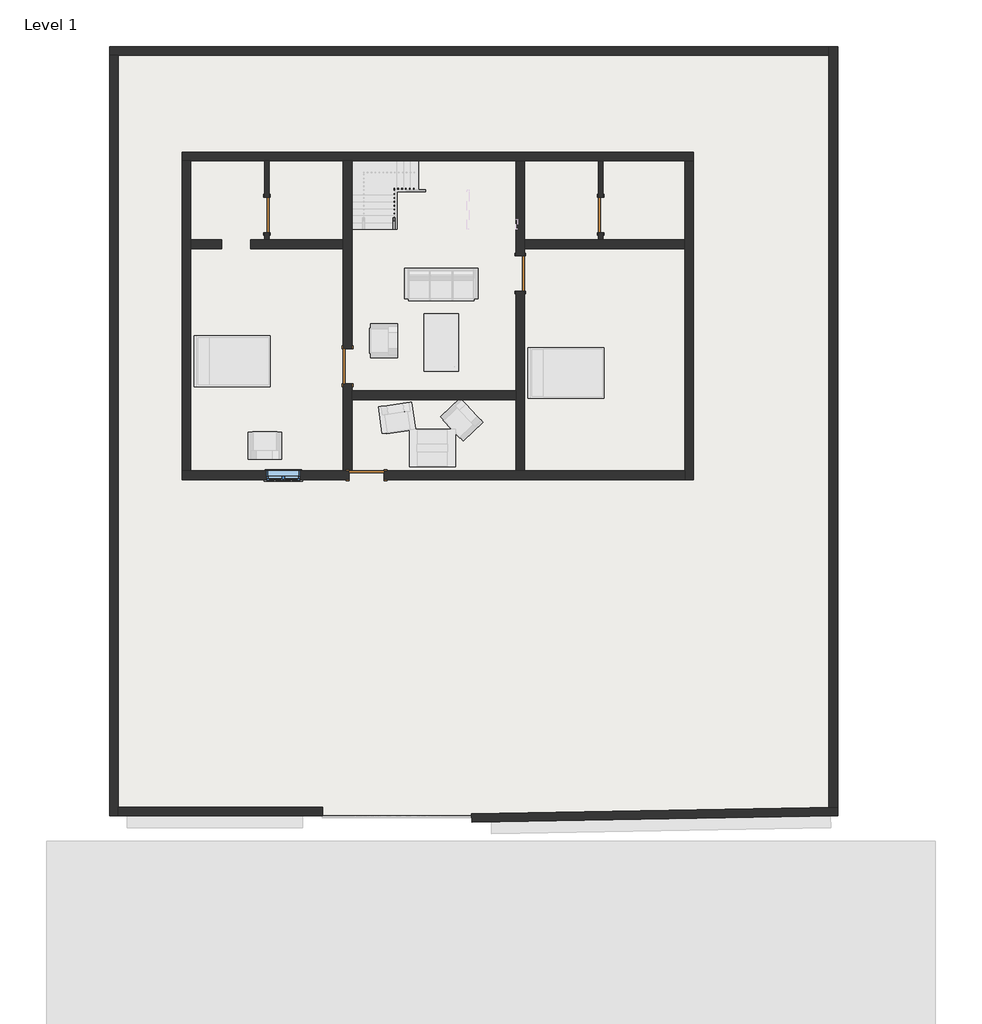
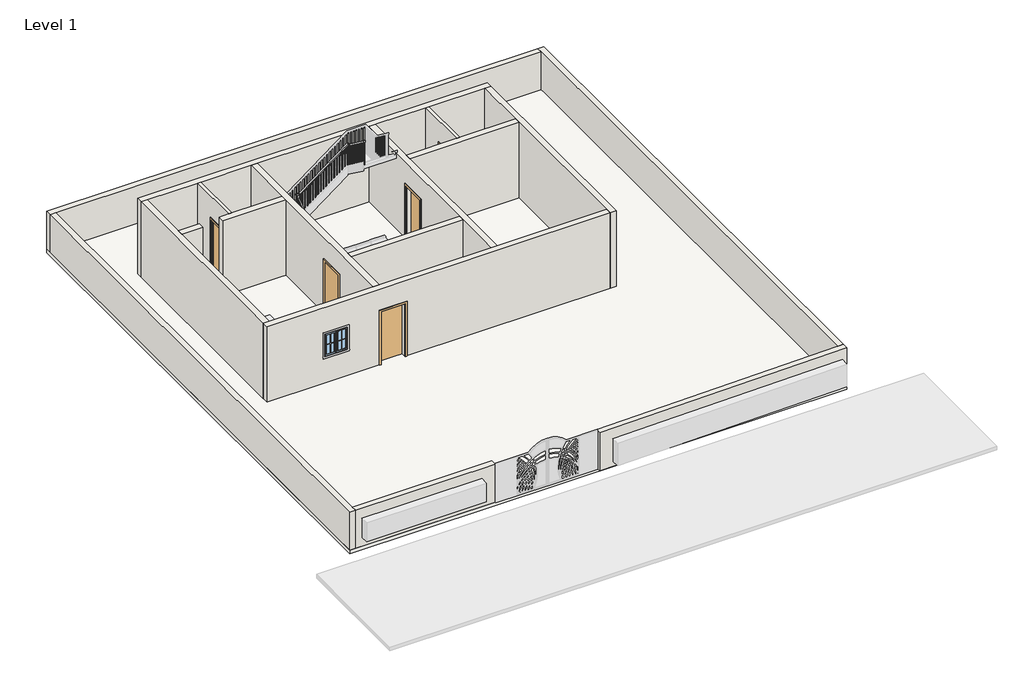
# One storey, part 1 of 2: 17 walls, 5 doors, 1 railing, 1 slab, 1 window.
"""IFC4 building model written with IfcOpenShell, lengths in millimetres."""

from ifc_helpers import new_model, si_unit, frame, origin, origin_with_axes, place, context, project, spatial, polyline, outline, extrude, faceted_brep, transform, mapped, element, save
from components import door_e5f9f3c4, door_a90ba1ad, door_305aa2a5, window_339605e1

model = new_model("IFC4")

# Units and contexts
model_context = context("Model", 3, world=origin())
ifc_project = project(units=[si_unit("LENGTHUNIT", "METRE", prefix="MILLI")], contexts=[model_context])

# Site, building, storey
site = spatial("IfcSite", under=ifc_project)
building = spatial("IfcBuilding", under=site)
storey = spatial("IfcBuildingStorey", under=building, Name="Level 1", Elevation=0.0)

# Doors
placement = place(None, origin())
door_shape = door_e5f9f3c4(model_context)
element("IfcDoor", 1, ObjectType="Single-Flush : 36\" x 84\"", at=placement, inside=storey, context=model_context, shape_type="MappedRepresentation", body=[
    mapped(door_shape, transform((-5709.1546642, 5087.2167606, 0.0), x_axis=(0.0, -1.0, 0.0), y_axis=(1.0, 0.0, 0.0), z_axis=(0.0, 0.0, 1.0))),
])
door_2_shape = door_a90ba1ad(model_context)
element("IfcDoor", 2, ObjectType="Single-Flush : 36\" x 84\"", at=placement, inside=storey, context=model_context, shape_type="MappedRepresentation", body=[
    mapped(door_2_shape, transform((-3607.3046642, 1150.2167606, 0.0), x_axis=(0.0, -1.0, 0.0), y_axis=(1.0, 0.0, 0.0), z_axis=(0.0, 0.0, 1.0))),
])
element("IfcDoor", 3, ObjectType="Single-Flush : 36\" x 84\"", at=placement, inside=storey, context=model_context, shape_type="MappedRepresentation", body=[
    mapped(door_2_shape, transform((888.4953358, 3563.2167606, 0.0), x_axis=(0.0, 1.0, 0.0), y_axis=(-1.0, 0.0, 0.0), z_axis=(0.0, 0.0, 1.0))),
])
element("IfcDoor", 4, ObjectType="Single-Flush : 36\" x 84\"", at=placement, inside=storey, context=model_context, shape_type="MappedRepresentation", body=[
    mapped(door_2_shape, transform((-3112.0046642, -1694.5832394, 0.0), x_axis=(-1.0, 0.0, 0.0), y_axis=(0.0, -1.0, 0.0), z_axis=(0.0, 0.0, 1.0))),
])
door_3_shape = door_305aa2a5(model_context)
element("IfcDoor", 5, ObjectType="Single-Flush : 36\" x 84\"", at=placement, inside=storey, context=model_context, shape_type="MappedRepresentation", body=[
    mapped(door_3_shape, transform((2990.3453358, 5087.2167606, 0.0), x_axis=(0.0, -1.0, 0.0), y_axis=(1.0, 0.0, 0.0), z_axis=(0.0, 0.0, 1.0))),
])

# Railing
element("IfcRailing", 6, ObjectType="Handrail - Rectangular", at=placement, inside=storey, context=model_context, shape_type="SolidModel", body=[
    faceted_brep([(-2419.4972892, 4718.9167606, 1046.9217391), (-2419.4972892, 4718.9167606, 983.5634439), (-2368.6972892, 4718.9167606, 983.5634439), (-2368.6972892, 4718.9167606, 1046.9217391), (-2419.4972892, 5670.3536537, 1756.0672495), (-2419.4972892, 5721.1536537, 1730.5723083), (-2368.6972892, 5721.1536537, 1730.5723083), (-2368.6972892, 5670.3536537, 1756.0672495), (-2419.4972892, 5670.3536537, 1862.8733611), (-2419.4972892, 5721.1536537, 1812.0733611), (-2368.6972892, 5721.1536537, 1812.0733611), (-2368.6972892, 5670.3536537, 1862.8733611), (-2419.4972892, 5797.3536537, 1862.8733611), (-2419.4972892, 5797.3536537, 1812.0733611), (-2368.6972892, 5746.5536537, 1812.0733611), (-2368.6972892, 5746.5536537, 1862.8733611), (-2292.4972892, 5797.3536537, 1862.8733611), (-2275.6482431, 5797.3536537, 1812.0733611), (-2275.6482431, 5746.5536537, 1812.0733611), (-2292.4972892, 5746.5536537, 1862.8733611), (-474.1369697, 5797.3536537, 3218.1729781), (-457.2879235, 5797.3536537, 3167.3729781), (-457.2879235, 5746.5536537, 3167.3729781), (-474.1369697, 5746.5536537, 3218.1729781), (-394.2046642, 5797.3536537, 3218.1729781), (-394.2046642, 5797.3536537, 3167.3729781), (-445.0046642, 5746.5536537, 3167.3729781), (-445.0046642, 5746.5536537, 3218.1729781), (-394.2046642, 5717.4213483, 3218.1729781), (-394.2046642, 5700.5723021, 3167.3729781), (-445.0046642, 5700.5723021, 3167.3729781), (-445.0046642, 5717.4213483, 3218.1729781), (-394.2046642, 4718.9167606, 3962.4), (-445.0046642, 4718.9167606, 3962.4), (-445.0046642, 4718.9167606, 3899.0417047), (-394.2046642, 4718.9167606, 3899.0417047)], [[[0, 1, 2, 3]], [[1, 0, 4, 5]], [[2, 1, 5, 6]], [[3, 2, 6, 7]], [[0, 3, 7, 4]], [[5, 4, 8, 9]], [[6, 5, 9, 10]], [[7, 6, 10, 11]], [[4, 7, 11, 8]], [[9, 8, 12, 13]], [[10, 9, 13, 14]], [[11, 10, 14, 15]], [[8, 11, 15, 12]], [[13, 12, 16, 17]], [[14, 13, 17, 18]], [[15, 14, 18, 19]], [[12, 15, 19, 16]], [[17, 16, 20, 21]], [[18, 17, 21, 22]], [[19, 18, 22, 23]], [[16, 19, 23, 20]], [[21, 20, 24, 25]], [[22, 21, 25, 26]], [[23, 22, 26, 27]], [[20, 23, 27, 24]], [[25, 24, 28, 29]], [[26, 25, 29, 30]], [[27, 26, 30, 31]], [[24, 27, 31, 28]], [[32, 33, 34, 35]], [[29, 28, 32, 35]], [[30, 29, 35, 34]], [[31, 30, 34, 33]], [[28, 31, 33, 32]]]),
    extrude(outline(polyline([(4746.4286537, 3878.5359459), (4765.4786537, 3864.3371882), (4765.4786537, 2915.4782609), (4746.4286537, 2915.4782609), (4746.4286537, 3878.5359459)])), frame((-429.1296642, 0.0, 0.0), z_axis=(1.0, 0.0, 0.0), x_axis=(0.0, 1.0, 0.0)), (0.0, 0.0, 1.0), 19.05),
    extrude(outline(polyline([(4848.0286537, 3802.8092378), (4867.0786537, 3788.6104801), (4867.0786537, 2915.4782609), (4848.0286537, 2915.4782609), (4848.0286537, 3802.8092378)])), frame((-429.1296642, 0.0, 0.0), z_axis=(1.0, 0.0, 0.0), x_axis=(0.0, 1.0, 0.0)), (0.0, 0.0, 1.0), 19.05),
    extrude(outline(polyline([(4949.6286537, 3727.0825298), (4968.6786537, 3712.883772), (4968.6786537, 2782.9565217), (4949.6286537, 2782.9565217), (4949.6286537, 3727.0825298)])), frame((-429.1296642, 0.0, 0.0), z_axis=(1.0, 0.0, 0.0), x_axis=(0.0, 1.0, 0.0)), (0.0, 0.0, 1.0), 19.05),
    extrude(outline(polyline([(5051.2286537, 3651.3558217), (5070.2786537, 3637.1570639), (5070.2786537, 2782.9565217), (5051.2286537, 2782.9565217), (5051.2286537, 3651.3558217)])), frame((-429.1296642, 0.0, 0.0), z_axis=(1.0, 0.0, 0.0), x_axis=(0.0, 1.0, 0.0)), (0.0, 0.0, 1.0), 19.05),
    extrude(outline(polyline([(5152.8286537, 3575.6291136), (5171.8786537, 3561.4303559), (5171.8786537, 2650.4347826), (5152.8286537, 2650.4347826), (5152.8286537, 3575.6291136)])), frame((-429.1296642, 0.0, 0.0), z_axis=(1.0, 0.0, 0.0), x_axis=(0.0, 1.0, 0.0)), (0.0, 0.0, 1.0), 19.05),
    extrude(outline(polyline([(5254.4286537, 3499.9024055), (5273.4786537, 3485.7036478), (5273.4786537, 2517.9130435), (5254.4286537, 2517.9130435), (5254.4286537, 3499.9024055)])), frame((-429.1296642, 0.0, 0.0), z_axis=(1.0, 0.0, 0.0), x_axis=(0.0, 1.0, 0.0)), (0.0, 0.0, 1.0), 19.05),
    extrude(outline(polyline([(5356.0286537, 3424.1756975), (5375.0786537, 3409.9769397), (5375.0786537, 2517.9130435), (5356.0286537, 2517.9130435), (5356.0286537, 3424.1756975)])), frame((-429.1296642, 0.0, 0.0), z_axis=(1.0, 0.0, 0.0), x_axis=(0.0, 1.0, 0.0)), (0.0, 0.0, 1.0), 19.05),
    extrude(outline(polyline([(5457.6286537, 3348.4489894), (5476.6786537, 3334.2502316), (5476.6786537, 2385.3913043), (5457.6286537, 2385.3913043), (5457.6286537, 3348.4489894)])), frame((-429.1296642, 0.0, 0.0), z_axis=(1.0, 0.0, 0.0), x_axis=(0.0, 1.0, 0.0)), (0.0, 0.0, 1.0), 19.05),
    extrude(outline(polyline([(5559.2286537, 3272.7222813), (5578.2786537, 3258.5235236), (5578.2786537, 2385.3913043), (5559.2286537, 2385.3913043), (5559.2286537, 3272.7222813)])), frame((-429.1296642, 0.0, 0.0), z_axis=(1.0, 0.0, 0.0), x_axis=(0.0, 1.0, 0.0)), (0.0, 0.0, 1.0), 19.05),
    extrude(outline(polyline([(5660.8286537, 3196.9955732), (5679.8786537, 3182.7968155), (5679.8786537, 2252.8695652), (5660.8286537, 2252.8695652), (5660.8286537, 3196.9955732)])), frame((-429.1296642, 0.0, 0.0), z_axis=(1.0, 0.0, 0.0), x_axis=(0.0, 1.0, 0.0)), (0.0, 0.0, 1.0), 19.05),
    extrude(outline(polyline([(-473.2222892, 5762.4286537), (-473.2222892, 5781.4786537), (-454.1722892, 5781.4786537), (-454.1722892, 5762.4286537), (-473.2222892, 5762.4286537)])), frame((0.0, 0.0, 2252.8695652), z_axis=(0.0, 0.0, 1.0), x_axis=(1.0, 0.0, 0.0)), (0.0, 0.0, 1.0), 914.5034129),
    extrude(outline(polyline([(3093.9684819, -555.7722892), (3079.7697242, -574.8222892), (2120.3478261, -574.8222892), (2120.3478261, -555.7722892), (3093.9684819, -555.7722892)])), frame((0.0, 5762.4286537, 0.0), z_axis=(0.0, 1.0, 0.0), x_axis=(0.0, 0.0, 1.0)), (0.0, 0.0, 1.0), 19.05),
    extrude(outline(polyline([(3018.2417739, -657.3722892), (3004.0430161, -676.4222892), (2120.3478261, -676.4222892), (2120.3478261, -657.3722892), (3018.2417739, -657.3722892)])), frame((0.0, 5762.4286537, 0.0), z_axis=(0.0, 1.0, 0.0), x_axis=(0.0, 0.0, 1.0)), (0.0, 0.0, 1.0), 19.05),
    extrude(outline(polyline([(2942.5150658, -758.9722892), (2928.316308, -778.0222892), (1987.826087, -778.0222892), (1987.826087, -758.9722892), (2942.5150658, -758.9722892)])), frame((0.0, 5762.4286537, 0.0), z_axis=(0.0, 1.0, 0.0), x_axis=(0.0, 0.0, 1.0)), (0.0, 0.0, 1.0), 19.05),
    extrude(outline(polyline([(2866.7883577, -860.5722892), (2852.5896, -879.6222892), (1987.826087, -879.6222892), (1987.826087, -860.5722892), (2866.7883577, -860.5722892)])), frame((0.0, 5762.4286537, 0.0), z_axis=(0.0, 1.0, 0.0), x_axis=(0.0, 0.0, 1.0)), (0.0, 0.0, 1.0), 19.05),
    extrude(outline(polyline([(2791.0616496, -962.1722892), (2776.8628919, -981.2222892), (1855.3043478, -981.2222892), (1855.3043478, -962.1722892), (2791.0616496, -962.1722892)])), frame((0.0, 5762.4286537, 0.0), z_axis=(0.0, 1.0, 0.0), x_axis=(0.0, 0.0, 1.0)), (0.0, 0.0, 1.0), 19.05),
    extrude(outline(polyline([(2715.3349416, -1063.7722892), (2701.1361838, -1082.8222892), (1855.3043478, -1082.8222892), (1855.3043478, -1063.7722892), (2715.3349416, -1063.7722892)])), frame((0.0, 5762.4286537, 0.0), z_axis=(0.0, 1.0, 0.0), x_axis=(0.0, 0.0, 1.0)), (0.0, 0.0, 1.0), 19.05),
    extrude(outline(polyline([(2639.6082335, -1165.3722892), (2625.4094757, -1184.4222892), (1722.7826087, -1184.4222892), (1722.7826087, -1165.3722892), (2639.6082335, -1165.3722892)])), frame((0.0, 5762.4286537, 0.0), z_axis=(0.0, 1.0, 0.0), x_axis=(0.0, 0.0, 1.0)), (0.0, 0.0, 1.0), 19.05),
    extrude(outline(polyline([(2563.8815254, -1266.9722892), (2549.6827677, -1286.0222892), (1590.2608696, -1286.0222892), (1590.2608696, -1266.9722892), (2563.8815254, -1266.9722892)])), frame((0.0, 5762.4286537, 0.0), z_axis=(0.0, 1.0, 0.0), x_axis=(0.0, 0.0, 1.0)), (0.0, 0.0, 1.0), 19.05),
    extrude(outline(polyline([(2488.1548173, -1368.5722892), (2473.9560596, -1387.6222892), (1590.2608696, -1387.6222892), (1590.2608696, -1368.5722892), (2488.1548173, -1368.5722892)])), frame((0.0, 5762.4286537, 0.0), z_axis=(0.0, 1.0, 0.0), x_axis=(0.0, 0.0, 1.0)), (0.0, 0.0, 1.0), 19.05),
    extrude(outline(polyline([(2412.4281093, -1470.1722892), (2398.2293515, -1489.2222892), (1457.7391304, -1489.2222892), (1457.7391304, -1470.1722892), (2412.4281093, -1470.1722892)])), frame((0.0, 5762.4286537, 0.0), z_axis=(0.0, 1.0, 0.0), x_axis=(0.0, 0.0, 1.0)), (0.0, 0.0, 1.0), 19.05),
    extrude(outline(polyline([(2336.7014012, -1571.7722892), (2322.5026434, -1590.8222892), (1457.7391304, -1590.8222892), (1457.7391304, -1571.7722892), (2336.7014012, -1571.7722892)])), frame((0.0, 5762.4286537, 0.0), z_axis=(0.0, 1.0, 0.0), x_axis=(0.0, 0.0, 1.0)), (0.0, 0.0, 1.0), 19.05),
    extrude(outline(polyline([(2260.9746931, -1673.3722892), (2246.7759354, -1692.4222892), (1325.2173913, -1692.4222892), (1325.2173913, -1673.3722892), (2260.9746931, -1673.3722892)])), frame((0.0, 5762.4286537, 0.0), z_axis=(0.0, 1.0, 0.0), x_axis=(0.0, 0.0, 1.0)), (0.0, 0.0, 1.0), 19.05),
    extrude(outline(polyline([(2185.247985, -1774.9722892), (2171.0492273, -1794.0222892), (1325.2173913, -1794.0222892), (1325.2173913, -1774.9722892), (2185.247985, -1774.9722892)])), frame((0.0, 5762.4286537, 0.0), z_axis=(0.0, 1.0, 0.0), x_axis=(0.0, 0.0, 1.0)), (0.0, 0.0, 1.0), 19.05),
    extrude(outline(polyline([(2109.521277, -1876.5722892), (2095.3225192, -1895.6222892), (1192.6956522, -1895.6222892), (1192.6956522, -1876.5722892), (2109.521277, -1876.5722892)])), frame((0.0, 5762.4286537, 0.0), z_axis=(0.0, 1.0, 0.0), x_axis=(0.0, 0.0, 1.0)), (0.0, 0.0, 1.0), 19.05),
    extrude(outline(polyline([(2033.7945689, -1978.1722892), (2019.5958111, -1997.2222892), (1060.173913, -1997.2222892), (1060.173913, -1978.1722892), (2033.7945689, -1978.1722892)])), frame((0.0, 5762.4286537, 0.0), z_axis=(0.0, 1.0, 0.0), x_axis=(0.0, 0.0, 1.0)), (0.0, 0.0, 1.0), 19.05),
    extrude(outline(polyline([(1958.0678608, -2079.7722892), (1943.8691031, -2098.8222892), (1060.173913, -2098.8222892), (1060.173913, -2079.7722892), (1958.0678608, -2079.7722892)])), frame((0.0, 5762.4286537, 0.0), z_axis=(0.0, 1.0, 0.0), x_axis=(0.0, 0.0, 1.0)), (0.0, 0.0, 1.0), 19.05),
    extrude(outline(polyline([(1882.3411527, -2181.3722892), (1868.142395, -2200.4222892), (927.6521739, -2200.4222892), (927.6521739, -2181.3722892), (1882.3411527, -2181.3722892)])), frame((0.0, 5762.4286537, 0.0), z_axis=(0.0, 1.0, 0.0), x_axis=(0.0, 0.0, 1.0)), (0.0, 0.0, 1.0), 19.05),
    extrude(outline(polyline([(1806.6144447, -2282.9722892), (1792.4156869, -2302.0222892), (927.6521739, -2302.0222892), (927.6521739, -2282.9722892), (1806.6144447, -2282.9722892)])), frame((0.0, 5762.4286537, 0.0), z_axis=(0.0, 1.0, 0.0), x_axis=(0.0, 0.0, 1.0)), (0.0, 0.0, 1.0), 19.05),
    extrude(outline(polyline([(-2384.5722892, 5725.3917606), (-2403.6222892, 5725.3917606), (-2403.6222892, 5744.4417606), (-2384.5722892, 5744.4417606), (-2384.5722892, 5725.3917606)])), frame((0.0, 0.0, 795.1304348), z_axis=(0.0, 0.0, 1.0), x_axis=(1.0, 0.0, 0.0)), (0.0, 0.0, 1.0), 1016.9429263),
    extrude(outline(polyline([(5623.7917606, 1658.0044377), (5642.8417606, 1672.2031954), (5642.8417606, 795.1304348), (5623.7917606, 795.1304348), (5623.7917606, 1658.0044377)])), frame((-2403.6222892, 0.0, 0.0), z_axis=(1.0, 0.0, 0.0), x_axis=(0.0, 1.0, 0.0)), (0.0, 0.0, 1.0), 19.05),
    extrude(outline(polyline([(5522.1917606, 1582.2777296), (5541.2417606, 1596.4764873), (5541.2417606, 662.6086957), (5522.1917606, 662.6086957), (5522.1917606, 1582.2777296)])), frame((-2403.6222892, 0.0, 0.0), z_axis=(1.0, 0.0, 0.0), x_axis=(0.0, 1.0, 0.0)), (0.0, 0.0, 1.0), 19.05),
    extrude(outline(polyline([(5420.5917606, 1506.5510215), (5439.6417606, 1520.7497793), (5439.6417606, 662.6086957), (5420.5917606, 662.6086957), (5420.5917606, 1506.5510215)])), frame((-2403.6222892, 0.0, 0.0), z_axis=(1.0, 0.0, 0.0), x_axis=(0.0, 1.0, 0.0)), (0.0, 0.0, 1.0), 19.05),
    extrude(outline(polyline([(5318.9917606, 1430.8243134), (5338.0417606, 1445.0230712), (5338.0417606, 530.0869565), (5318.9917606, 530.0869565), (5318.9917606, 1430.8243134)])), frame((-2403.6222892, 0.0, 0.0), z_axis=(1.0, 0.0, 0.0), x_axis=(0.0, 1.0, 0.0)), (0.0, 0.0, 1.0), 19.05),
    extrude(outline(polyline([(5217.3917606, 1355.0976054), (5236.4417606, 1369.2963631), (5236.4417606, 397.5652174), (5217.3917606, 397.5652174), (5217.3917606, 1355.0976054)])), frame((-2403.6222892, 0.0, 0.0), z_axis=(1.0, 0.0, 0.0), x_axis=(0.0, 1.0, 0.0)), (0.0, 0.0, 1.0), 19.05),
    extrude(outline(polyline([(5115.7917606, 1279.3708973), (5134.8417606, 1293.569655), (5134.8417606, 397.5652174), (5115.7917606, 397.5652174), (5115.7917606, 1279.3708973)])), frame((-2403.6222892, 0.0, 0.0), z_axis=(1.0, 0.0, 0.0), x_axis=(0.0, 1.0, 0.0)), (0.0, 0.0, 1.0), 19.05),
    extrude(outline(polyline([(5014.1917606, 1203.6441892), (5033.2417606, 1217.842947), (5033.2417606, 265.0434783), (5014.1917606, 265.0434783), (5014.1917606, 1203.6441892)])), frame((-2403.6222892, 0.0, 0.0), z_axis=(1.0, 0.0, 0.0), x_axis=(0.0, 1.0, 0.0)), (0.0, 0.0, 1.0), 19.05),
    extrude(outline(polyline([(4912.5917606, 1127.9174811), (4931.6417606, 1142.1162389), (4931.6417606, 265.0434783), (4912.5917606, 265.0434783), (4912.5917606, 1127.9174811)])), frame((-2403.6222892, 0.0, 0.0), z_axis=(1.0, 0.0, 0.0), x_axis=(0.0, 1.0, 0.0)), (0.0, 0.0, 1.0), 19.05),
    extrude(outline(polyline([(4810.9917606, 1052.1907731), (4830.0417606, 1066.3895308), (4830.0417606, 132.5217391), (4810.9917606, 132.5217391), (4810.9917606, 1052.1907731)])), frame((-2403.6222892, 0.0, 0.0), z_axis=(1.0, 0.0, 0.0), x_axis=(0.0, 1.0, 0.0)), (0.0, 0.0, 1.0), 19.05),
    extrude(outline(polyline([(-429.1296642, 5762.4286537), (-429.1296642, 5781.4786537), (-410.0796642, 5781.4786537), (-410.0796642, 5762.4286537), (-429.1296642, 5762.4286537)])), frame((0.0, 0.0, 2252.8695652), z_axis=(0.0, 0.0, 1.0), x_axis=(1.0, 0.0, 0.0)), (0.0, 0.0, 1.0), 914.5034129),
    extrude(outline(polyline([(-2384.5722892, 5762.4286537), (-2403.6222892, 5762.4286537), (-2403.6222892, 5781.4786537), (-2384.5722892, 5781.4786537), (-2384.5722892, 5762.4286537)])), frame((0.0, 0.0, 795.1304348), z_axis=(0.0, 0.0, 1.0), x_axis=(1.0, 0.0, 0.0)), (0.0, 0.0, 1.0), 1016.9429263),
    extrude(outline(polyline([(4718.9167606, 3899.0417047), (4737.9667606, 3884.842947), (4737.9667606, 2915.4782609), (4718.9167606, 2915.4782609), (4718.9167606, 3899.0417047)])), frame((-429.1296642, 0.0, 0.0), z_axis=(1.0, 0.0, 0.0), x_axis=(0.0, 1.0, 0.0)), (0.0, 0.0, 1.0), 19.05),
    extrude(outline(polyline([(4718.9167606, 983.5634439), (4737.9667606, 997.7622016), (4737.9667606, 132.5217391), (4718.9167606, 132.5217391), (4718.9167606, 983.5634439)])), frame((-2403.6222892, 0.0, 0.0), z_axis=(1.0, 0.0, 0.0), x_axis=(0.0, 1.0, 0.0)), (0.0, 0.0, 1.0), 19.05),
])

# Slab
element("IfcSlab", 7, ObjectType="Generic - 12\"", at=placement, inside=storey, context=model_context, shape_type="SweptSolid", body=[
    extrude(outline(polyline([(9160.8873014, 9474.0019835), (9160.8873014, -10564.2895294), (-9812.9126986, -10564.2895294), (-9812.9126986, 9474.0019835), (9160.8873014, 9474.0019835)])), frame((0.0, 0.0, -152.4), z_axis=(0.0, 0.0, 1.0), x_axis=(1.0, 0.0, 0.0)), (0.0, 0.0, 1.0), 152.4),
])

# Walls
element("IfcWall", 8, ObjectType="WALL4.5\"", at=placement, inside=storey, context=model_context, shape_type="SweptSolid", body=[
    extrude(outline(polyline([(4630.0167606, 2133.6), (4630.0167606, 0.0), (4439.5167606, 0.0), (4439.5167606, 3048.0), (6496.9167606, 3048.0), (6496.9167606, 0.0), (5544.4167606, 0.0), (5544.4167606, 2133.6), (4630.0167606, 2133.6)])), frame((-5766.3046642, 0.0, 0.0), z_axis=(1.0, 0.0, 0.0), x_axis=(0.0, 1.0, 0.0)), (0.0, 0.0, 1.0), 114.3),
])
element("IfcWall", 9, ObjectType="WALL4.5\"", at=placement, inside=storey, context=model_context, shape_type="SweptSolid", body=[
    extrude(outline(polyline([(4630.0167606, 2133.6), (4630.0167606, 0.0), (4439.5167606, 0.0), (4439.5167606, 3048.0), (6496.9167606, 3048.0), (6496.9167606, 0.0), (5544.4167606, 0.0), (5544.4167606, 2133.6), (4630.0167606, 2133.6)])), frame((2933.1953358, 0.0, 0.0), z_axis=(1.0, 0.0, 0.0), x_axis=(0.0, 1.0, 0.0)), (0.0, 0.0, 1.0), 114.3),
])
element("IfcWall", 10, ObjectType="WALL9\"", at=placement, inside=storey, context=model_context, shape_type="Brep", body=[
    faceted_brep([(-7925.3046642, 6496.9167606, 0.0), (-7696.7046642, 6496.9167606, 0.0), (-5766.3046642, 6496.9167606, 0.0), (-5652.0046642, 6496.9167606, 0.0), (-3721.6046642, 6496.9167606, 0.0), (-3493.0046642, 6496.9167606, 0.0), (774.1953358, 6496.9167606, 0.0), (1002.7953358, 6496.9167606, 0.0), (2933.1953358, 6496.9167606, 0.0), (3047.4953358, 6496.9167606, 0.0), (5181.0953358, 6496.9167606, 0.0), (5409.6953358, 6496.9167606, 0.0), (5409.6953358, 6496.9167606, 3048.0), (5181.0953358, 6496.9167606, 3048.0), (3047.4953358, 6496.9167606, 3048.0), (2933.1953358, 6496.9167606, 3048.0), (1002.7953358, 6496.9167606, 3048.0), (774.1953358, 6496.9167606, 3048.0), (-3493.0046642, 6496.9167606, 3048.0), (-3721.6046642, 6496.9167606, 3048.0), (-5652.0046642, 6496.9167606, 3048.0), (-5766.3046642, 6496.9167606, 3048.0), (-7696.7046642, 6496.9167606, 3048.0), (-7925.3046642, 6496.9167606, 3048.0), (-7925.3046642, 6725.5167606, 0.0), (-7925.3046642, 6725.5167606, 3048.0), (5409.6953358, 6725.5167606, 3048.0), (5409.6953358, 6725.5167606, 0.0)], [[[0, 1, 2, 3, 4, 5, 6, 7, 8, 9, 10, 11, 12, 13, 14, 15, 16, 17, 18, 19, 20, 21, 22, 23]], [[24, 25, 26, 27]], [[11, 10, 9, 8, 7, 6, 5, 4, 3, 2, 1, 0, 24, 27]], [[12, 11, 27, 26]], [[0, 23, 25, 24]], [[23, 22, 21, 20, 19, 18, 17, 16, 15, 14, 13, 12, 26, 25]]]),
])
element("IfcWall", 11, ObjectType="WALL9\"", at=placement, inside=storey, context=model_context, shape_type="Brep", body=[
    faceted_brep([(5181.0953358, 6496.9167606, 0.0), (5181.0953358, 4439.5167606, 0.0), (5181.0953358, 4210.9167606, 0.0), (5181.0953358, -1580.2832394, 0.0), (5181.0953358, -1808.8832394, 0.0), (5181.0953358, -1808.8832394, 3048.0), (5181.0953358, -1580.2832394, 3048.0), (5181.0953358, 4210.9167606, 3048.0), (5181.0953358, 4439.5167606, 3048.0), (5181.0953358, 6496.9167606, 3048.0), (5409.6953358, 6496.9167606, 0.0), (5409.6953358, 6496.9167606, 3048.0), (5409.6953358, -1808.8832394, 3048.0), (5409.6953358, -1808.8832394, 0.0)], [[[0, 1, 2, 3, 4, 5, 6, 7, 8, 9]], [[10, 11, 12, 13]], [[4, 3, 2, 1, 0, 10, 13]], [[0, 9, 11, 10]], [[5, 4, 13, 12]], [[9, 8, 7, 6, 5, 12, 11]]]),
])
element("IfcWall", 12, ObjectType="WALL9\"", at=placement, inside=storey, context=model_context, shape_type="Brep", body=[
    faceted_brep([(-3569.2046642, -1580.2832394, 2133.6), (-3569.2046642, -1580.2832394, 0.0), (-3721.6046642, -1580.2832394, 0.0), (-7696.7046642, -1580.2832394, 0.0), (-7925.3046642, -1580.2832394, 0.0), (-7925.3046642, -1580.2832394, 3048.0), (-7696.7046642, -1580.2832394, 3048.0), (-3721.6046642, -1580.2832394, 3048.0), (-3493.0046642, -1580.2832394, 3048.0), (774.1953358, -1580.2832394, 3048.0), (1002.7953358, -1580.2832394, 3048.0), (5181.0953358, -1580.2832394, 3048.0), (5181.0953358, -1580.2832394, 0.0), (1002.7953358, -1580.2832394, 0.0), (774.1953358, -1580.2832394, 0.0), (-2654.8046642, -1580.2832394, 0.0), (-2654.8046642, -1580.2832394, 2133.6), (-5715.5046642, -1580.2832394, 1981.5434313), (-5715.5046642, -1580.2832394, 1067.1434313), (-4851.9046642, -1580.2832394, 1067.1434313), (-4851.9046642, -1580.2832394, 1981.5434313), (-7925.3046642, -1808.8832394, 0.0), (-3569.2046642, -1808.8832394, 0.0), (-3569.2046642, -1808.8832394, 2133.6), (-2654.8046642, -1808.8832394, 2133.6), (-2654.8046642, -1808.8832394, 0.0), (5181.0953358, -1808.8832394, 0.0), (5181.0953358, -1808.8832394, 3048.0), (-7925.3046642, -1808.8832394, 3048.0), (-5715.5046642, -1808.8832394, 1981.5434313), (-4851.9046642, -1808.8832394, 1981.5434313), (-4851.9046642, -1808.8832394, 1067.1434313), (-5715.5046642, -1808.8832394, 1067.1434313)], [[[0, 1, 2, 3, 4, 5, 6, 7, 8, 9, 10, 11, 12, 13, 14, 15, 16], [17, 18, 19, 20]], [[21, 22, 23, 24, 25, 26, 27, 28], [29, 30, 31, 32]], [[4, 3, 2, 1, 22, 21]], [[15, 14, 13, 12, 26, 25]], [[12, 11, 27, 26]], [[5, 4, 21, 28]], [[23, 22, 1, 0]], [[24, 23, 0, 16]], [[25, 24, 16, 15]], [[11, 10, 9, 8, 7, 6, 5, 28, 27]], [[18, 17, 29, 32]], [[19, 18, 32, 31]], [[20, 19, 31, 30]], [[17, 20, 30, 29]]]),
])
element("IfcWall", 13, ObjectType="WALL9\"", at=placement, inside=storey, context=model_context, shape_type="Brep", body=[
    faceted_brep([(-7696.7046642, -1580.2832394, 0.0), (-7696.7046642, 4210.9167606, 0.0), (-7696.7046642, 4439.5167606, 0.0), (-7696.7046642, 6496.9167606, 0.0), (-7696.7046642, 6496.9167606, 3048.0), (-7696.7046642, 4439.5167606, 3048.0), (-7696.7046642, 4210.9167606, 3048.0), (-7696.7046642, -1580.2832394, 3048.0), (-7925.3046642, -1580.2832394, 0.0), (-7925.3046642, -1580.2832394, 3048.0), (-7925.3046642, 6496.9167606, 3048.0), (-7925.3046642, 6496.9167606, 0.0)], [[[0, 1, 2, 3, 4, 5, 6, 7]], [[8, 9, 10, 11]], [[3, 2, 1, 0, 8, 11]], [[4, 3, 11, 10]], [[0, 7, 9, 8]], [[7, 6, 5, 4, 10, 9]]]),
])
element("IfcWall", 14, ObjectType="WALL9\"", at=placement, inside=storey, context=model_context, shape_type="Brep", body=[
    faceted_brep([(-3721.6046642, 693.0167606, 2133.6), (-3721.6046642, 693.0167606, 0.0), (-3721.6046642, -1580.2832394, 0.0), (-3721.6046642, -1580.2832394, 3048.0), (-3721.6046642, 4210.9167606, 3048.0), (-3721.6046642, 4439.5167606, 3048.0), (-3721.6046642, 6496.9167606, 3048.0), (-3721.6046642, 6496.9167606, 0.0), (-3721.6046642, 4439.5167606, 0.0), (-3721.6046642, 4210.9167606, 0.0), (-3721.6046642, 1607.4167606, 0.0), (-3721.6046642, 1607.4167606, 2133.6), (-3493.0046642, -1580.2832394, 0.0), (-3493.0046642, 273.9167606, 0.0), (-3493.0046642, 502.5167606, 0.0), (-3493.0046642, 693.0167606, 0.0), (-3493.0046642, 693.0167606, 2133.6), (-3493.0046642, 1607.4167606, 2133.6), (-3493.0046642, 1607.4167606, 0.0), (-3493.0046642, 6496.9167606, 0.0), (-3493.0046642, 6496.9167606, 3048.0), (-3493.0046642, 502.5167606, 3048.0), (-3493.0046642, 273.9167606, 3048.0), (-3493.0046642, -1580.2832394, 3048.0)], [[[0, 1, 2, 3, 4, 5, 6, 7, 8, 9, 10, 11]], [[12, 13, 14, 15, 16, 17, 18, 19, 20, 21, 22, 23]], [[2, 1, 15, 14, 13, 12]], [[10, 9, 8, 7, 19, 18]], [[7, 6, 20, 19]], [[3, 2, 12, 23]], [[16, 15, 1, 0]], [[17, 16, 0, 11]], [[18, 17, 11, 10]], [[6, 5, 4, 3, 23, 22, 21, 20]]]),
])
element("IfcWall", 15, ObjectType="WALL9\"", at=placement, inside=storey, context=model_context, shape_type="Brep", body=[
    faceted_brep([(774.1953358, 6496.9167606, 0.0), (774.1953358, 4020.4167606, 0.0), (774.1953358, 4020.4167606, 2133.6), (774.1953358, 3106.0167606, 2133.6), (774.1953358, 3106.0167606, 0.0), (774.1953358, 502.5167606, 0.0), (774.1953358, 273.9167606, 0.0), (774.1953358, -1580.2832394, 0.0), (774.1953358, -1580.2832394, 3048.0), (774.1953358, 273.9167606, 3048.0), (774.1953358, 502.5167606, 3048.0), (774.1953358, 4668.1167606, 3048.0), (774.1953358, 6446.1167606, 3048.0), (774.1953358, 6496.9167606, 3048.0), (1002.7953358, 4020.4167606, 2133.6), (1002.7953358, 4020.4167606, 0.0), (1002.7953358, 4210.9167606, 0.0), (1002.7953358, 4439.5167606, 0.0), (1002.7953358, 6496.9167606, 0.0), (1002.7953358, 6496.9167606, 3048.0), (1002.7953358, 4439.5167606, 3048.0), (1002.7953358, 4210.9167606, 3048.0), (1002.7953358, -1580.2832394, 3048.0), (1002.7953358, -1580.2832394, 0.0), (1002.7953358, 3106.0167606, 0.0), (1002.7953358, 3106.0167606, 2133.6)], [[[0, 1, 2, 3, 4, 5, 6, 7, 8, 9, 10, 11, 12, 13]], [[14, 15, 16, 17, 18, 19, 20, 21, 22, 23, 24, 25]], [[24, 23, 7, 6, 5, 4]], [[18, 17, 16, 15, 1, 0]], [[0, 13, 19, 18]], [[8, 7, 23, 22]], [[2, 1, 15, 14]], [[3, 2, 14, 25]], [[4, 3, 25, 24]], [[13, 12, 11, 10, 9, 8, 22, 21, 20, 19]]]),
])
element("IfcWall", 16, ObjectType="WALL9\"", at=placement, inside=storey, context=model_context, shape_type="SweptSolid", body=[
    extrude(outline(polyline([(774.1953358, 273.9167606), (-3493.0046642, 273.9167606), (-3493.0046642, 502.5167606), (774.1953358, 502.5167606), (774.1953358, 273.9167606)])), origin_with_axes(), (0.0, 0.0, 1.0), 3048.0),
])
element("IfcWall", 17, ObjectType="WALL9\"", at=placement, inside=storey, context=model_context, shape_type="SweptSolid", body=[
    extrude(outline(polyline([(-6895.4507894, 4210.9167606), (-7696.7046642, 4210.9167606), (-7696.7046642, 4439.5167606), (-6895.4507894, 4439.5167606), (-6895.4507894, 4210.9167606)])), origin_with_axes(), (0.0, 0.0, 1.0), 3048.0),
])
element("IfcWall", 18, ObjectType="WALL9\"", at=placement, inside=storey, context=model_context, shape_type="Brep", body=[
    faceted_brep([(-3721.6046642, 4439.5167606, 0.0), (-5652.0046642, 4439.5167606, 0.0), (-5766.3046642, 4439.5167606, 0.0), (-6131.0963491, 4439.5167606, 0.0), (-6131.0963491, 4439.5167606, 3048.0), (-5766.3046642, 4439.5167606, 3048.0), (-5652.0046642, 4439.5167606, 3048.0), (-3721.6046642, 4439.5167606, 3048.0), (-3721.6046642, 4210.9167606, 0.0), (-3721.6046642, 4210.9167606, 3048.0), (-6131.0963491, 4210.9167606, 3048.0), (-6131.0963491, 4210.9167606, 0.0)], [[[0, 1, 2, 3, 4, 5, 6, 7]], [[8, 9, 10, 11]], [[3, 2, 1, 0, 8, 11]], [[4, 3, 11, 10]], [[0, 7, 9, 8]], [[7, 6, 5, 4, 10, 9]]]),
])
element("IfcWall", 19, ObjectType="WALL9\"", at=placement, inside=storey, context=model_context, shape_type="Brep", body=[
    faceted_brep([(1002.7953358, 4210.9167606, 0.0), (5181.0953358, 4210.9167606, 0.0), (5181.0953358, 4210.9167606, 3048.0), (1002.7953358, 4210.9167606, 3048.0), (1002.7953358, 4439.5167606, 0.0), (1002.7953358, 4439.5167606, 3048.0), (2933.1953358, 4439.5167606, 3048.0), (3047.4953358, 4439.5167606, 3048.0), (5181.0953358, 4439.5167606, 3048.0), (5181.0953358, 4439.5167606, 0.0), (3047.4953358, 4439.5167606, 0.0), (2933.1953358, 4439.5167606, 0.0)], [[[0, 1, 2, 3]], [[4, 5, 6, 7, 8, 9, 10, 11]], [[1, 0, 4, 11, 10, 9]], [[2, 1, 9, 8]], [[0, 3, 5, 4]], [[3, 2, 8, 7, 6, 5]]]),
])
element("IfcWall", 20, ObjectType="WALL9\"", at=placement, inside=storey, context=model_context, shape_type="Brep", body=[
    faceted_brep([(-9812.9126986, 9245.4019835, 0.0), (-9584.3126986, 9245.4019835, 0.0), (8932.2873014, 9245.4019835, 0.0), (8932.2873014, 9245.4019835, 1524.0), (-9584.3126986, 9245.4019835, 1524.0), (-9812.9126986, 9245.4019835, 1524.0), (-9812.9126986, 9474.0019835, 0.0), (-9812.9126986, 9474.0019835, 1524.0), (8932.2873014, 9474.0019835, 1524.0), (8932.2873014, 9474.0019835, 0.0)], [[[0, 1, 2, 3, 4, 5]], [[6, 7, 8, 9]], [[2, 1, 0, 6, 9]], [[5, 4, 3, 8, 7]], [[0, 5, 7, 6]], [[3, 2, 9, 8]]]),
])
element("IfcWall", 21, ObjectType="WALL9\"", at=placement, inside=storey, context=model_context, shape_type="Brep", body=[
    faceted_brep([(-9584.3126986, -10566.5980165, 0.0), (-9584.3126986, -10337.9980165, 0.0), (-9584.3126986, 9245.4019835, 0.0), (-9584.3126986, 9245.4019835, 1524.0), (-9584.3126986, -10337.9980165, 1524.0), (-9584.3126986, -10566.5980165, 1524.0), (-9812.9126986, -10566.5980165, 0.0), (-9812.9126986, -10566.5980165, 1524.0), (-9812.9126986, 9245.4019835, 1524.0), (-9812.9126986, 9245.4019835, 0.0)], [[[0, 1, 2, 3, 4, 5]], [[6, 7, 8, 9]], [[2, 1, 0, 6, 9]], [[5, 4, 3, 8, 7]], [[0, 5, 7, 6]], [[3, 2, 9, 8]]]),
])
element("IfcWall", 22, ObjectType="WALL9\"", at=placement, inside=storey, context=model_context, shape_type="Brep", body=[
    faceted_brep([(9160.8873014, -10336.0029026, 0.0), (8932.2873014, -10339.9931304, 0.0), (-375.3774692, -10502.4590233, 0.0), (-375.3774692, -10502.4590233, 1524.0), (8932.2873014, -10339.9931304, 1524.0), (9160.8873014, -10336.0029026, 1524.0), (9160.8873014, -10564.6377247, 0.0), (9160.8873014, -10564.6377247, 1524.0), (-371.3878491, -10731.0242064, 1524.0), (-371.3878491, -10731.0242064, 0.0)], [[[0, 1, 2, 3, 4, 5]], [[6, 7, 8, 9]], [[2, 1, 0, 6, 9]], [[3, 2, 9, 8]], [[5, 4, 3, 8, 7]], [[0, 5, 7, 6]]]),
])
element("IfcWall", 23, ObjectType="WALL9\"", at=placement, inside=storey, context=model_context, shape_type="Brep", body=[
    faceted_brep([(8932.2873014, 9474.0019835, 0.0), (8932.2873014, 9245.4019835, 0.0), (8932.2873014, -10339.9931304, 0.0), (8932.2873014, -10339.9931304, 1524.0), (8932.2873014, 9245.4019835, 1524.0), (8932.2873014, 9474.0019835, 1524.0), (9160.8873014, 9474.0019835, 0.0), (9160.8873014, 9474.0019835, 1524.0), (9160.8873014, -10336.0029026, 1524.0), (9160.8873014, -10336.0029026, 0.0)], [[[0, 1, 2, 3, 4, 5]], [[6, 7, 8, 9]], [[2, 1, 0, 6, 9]], [[5, 4, 3, 8, 7]], [[0, 5, 7, 6]], [[3, 2, 9, 8]]]),
])
element("IfcWall", 24, ObjectType="WALL9\"", at=placement, inside=storey, context=model_context, shape_type="SweptSolid", body=[
    extrude(outline(polyline([(-9584.3126986, -10337.9980165), (-4263.0126986, -10337.9980165), (-4263.0126986, -10566.5980165), (-9584.3126986, -10566.5980165), (-9584.3126986, -10337.9980165)])), origin_with_axes(), (0.0, 0.0, 1.0), 1524.0),
])

# Window
window_shape = window_339605e1(model_context)
element("IfcWindow", 25, ObjectType="Window-Casement-Double : 34\" x 36\"", at=placement, inside=storey, context=model_context, shape_type="MappedRepresentation", body=[
    mapped(window_shape, transform((-5283.7046642, -1694.5832394, 152.7434313), x_axis=(-1.0, 0.0, 0.0), y_axis=(0.0, -1.0, 0.0), z_axis=(0.0, 0.0, 1.0))),
])

save(model, "model.ifc")

# Revit data of these elements
# Type "Single-Flush : 36\" x 84\""
#   Type Mark = "1"
#   Construction Type Id = "MDOOR"
#   Assembly Code = "C1020"
#   Analytic Construction = "Metal"
#   Thickness = 0' - 2"
#   Heat Transfer Coefficient (U) = 0.651978 BTU/(h·ft²·°F)
#   Height = 7' - 0"
#   Trim Projection Ext = 0' - 1"
#   Trim Projection Int = 0' - 1"
#   Trim Width = 0' - 3"
#   Width = 3' - 0"
#   Define Thermal Properties by = 1
#   Define Thermal Properties by = 1
#   Door Material = Door - Panel
#   Frame Material = Door - Frame
#   Visual Light Transmittance = 0
#   Solar Heat Gain Coefficient = 0
#   Function = (empty or 0)
#   Wall Closure = (empty or 0)
# Type "Handrail - Rectangular"
#   Assembly Code = "C2010400"
#   built-in parameter 1008612 = 0.0416667 (stored number, unit not read)
#   built-in parameter 1008611 = 0.0416667 (stored number, unit not read)
#   built-in parameter 1008609 = 0.333333 (stored number, unit not read)
#   built-in parameter 1008604 = 0.166667 (stored number, unit not read)
#   built-in parameter 1008603 = 0.166667 (stored number, unit not read)
#   Railing Height = 3' - 0"
#   built-in parameter 1008630 = 2
#   built-in parameter 1008610 = 2
#   built-in parameter 1008618 = Baluster - Square : 3/4"
# Type "Generic - 12\""
#   Assembly Code = "B1010"
#   Function = 0
#   Layers, outside or top first: 0' - 6" no material (function 1)
# Type "WALL4.5\""
#   Assembly Code = "B2010"
#   Layers, outside or top first: 0' - 4 1/2" no material (function 1)
# Type "WALL9\""
#   Assembly Code = "B2010"
#   Layers, outside or top first: 0' - 9" no material (function 1)
# Type "Window-Casement-Double : 34\" x 36\""
#   Type Mark = "14"
#   Fire Rating = "0.5h"
#   Assembly Code = "B2020100"
#   Analytic Construction = "Double glazing - domestic"
#   Frame Extension [instance default] = 0' - 0 1/4"
#   Window Inset [instance default] = 0' - 0"
#   Wall Thickness [instance default] = 0' - 6"
#   Interior Wall Closure [instance default] = 0' - 2 1/4"
#   Half Width = 1' - 5"
#   Visual Light Transmittance = 0.81
#   Thermal Resistance (R) = 1.8146 (h·ft²·°F)/BTU
#   Solar Heat Gain Coefficient = 0.76
#   Rough Width = 2' - 10 1/2"
#   Rough Height = 3' - 0 1/2"
#   Height = 3' - 0"
#   Heat Transfer Coefficient (U) = 0.5511 BTU/(h·ft²·°F)
#   Exterior Wall Closure [instance default] = 0' - 1 1/4"
#   Extension Jamb [instance default] = 0' - 2 1/4"
#   Default Sill Height = 3' - 0"
#   Width = 2' - 10"
#   Define Thermal Properties by = 0
#   Muntin Visibility = yes
#   Interior Trim Visibility [instance default] = yes
#   Exterior Trim Visibility [instance default] = yes
#   Extension Jamb Visibility [instance default] = yes
#   Interior Trim Material = Wood - Stained
#   Muntin Pattern = Muntin Pattern_2x2 : Muntin Pattern_2x2
#   Interior Trim = Trim-Window-Interior-Flat : Picture Frame
#   Interior Frame Material = Wood - Stained
#   Glass Panel Material = Glass
#   Exterior Trim Material = Clad - White
#   Exterior Trim = Trim-Window-Exterior-Flat : with Sill
#   Exterior Frame Material = Clad - White
#   Wall Closure = (empty or 0)
# Elements 1, 2, 3, 4, 5 (IfcDoor, "Single-Flush : 36\" x 84\"")
#   Phase Created = New Construction
#   Materials on its faces: "Door - Frame", "Door - Panel"
# Element 6 (IfcRailing, "Handrail - Rectangular")
#   Phase Created = New Construction
# Element 7 (IfcSlab, "Generic - 12\"")
#   Height Offset From Level = 0' - 0"
#   Phase Created = New Construction
#   Materials on its faces: "Default Floor", "TI"
# Elements 8, 9 (IfcWall, "WALL4.5\"")
#   Top Offset = 0' - 0"
#   Base Offset = 0' - 0"
#   Unconnected Height = 10' - 0"
#   wall height = 10' - 0"
#   Phase Created = New Construction
#   Base Constraint = Level 1
#   Materials on its faces: "Default Wall"
# Elements 10, 11, 12, 13, 14, 15, 16, 17, 18, 19 (IfcWall, "WALL9\"")
#   Top Offset = 0' - 0"
#   Base Offset = 0' - 0"
#   Unconnected Height = 10' - 0"
#   wall height = 10' - 0"
#   Phase Created = New Construction
#   Base Constraint = Level 1
#   Materials on its faces: "Default Wall"
# Element 20 (IfcWall, "WALL9\"")
#   Top Offset = 0' - 0"
#   Base Offset = 0' - 0"
#   Unconnected Height = 5' - 0"
#   wall height = 5' - 0"
#   Phase Created = New Construction
#   Base Constraint = Level 1
#   Materials on its faces: "Default Wall", "Wood - Stained", "TTT"
# Elements 21, 22, 23, 24 (IfcWall, "WALL9\"")
#   Top Offset = 0' - 0"
#   Base Offset = 0' - 0"
#   Unconnected Height = 5' - 0"
#   wall height = 5' - 0"
#   Phase Created = New Construction
#   Base Constraint = Level 1
#   Materials on its faces: "Default Wall", "Wood - Stained"
# Element 25 (IfcWindow, "Window-Casement-Double : 34\" x 36\"")
#   Mark = "1"
#   Window Inset = 0' - 0"
#   Interior Wall Closure = 0' - 2 1/4"
#   Frame Extension = 0' - 0 1/4"
#   Exterior Wall Closure = 0' - 1 1/4"
#   Interior Trim Visibility = yes
#   Exterior Trim Visibility = yes
#   Phase Created = New Construction
#   Materials on its faces: "Wood - Stained", "Glass", "Clad - White"
# Materials
#   "Door - Panel": class "Wood", colour RGB 210 159 95, transparency 0, Cost = 0
#   "Door - Frame": colour RGB 118 70 51, transparency 0, Cost = 0
#   "Wood - Stained": class "Wood", colour RGB 224 178 126, transparency 0, Cost = 0
#   "Glass": class "Glass", colour RGB 0 128 192, transparency 0.75, Description = "Soda Lime Glass", Cost = 0
#   "Clad - White": class "Wood", colour RGB 242 242 238, transparency 0, Cost = 0
#   "Default Floor": colour RGB 128 128 128, transparency 0, Cost = 0
#   "TI": class "Generic", colour RGB 120 120 120, transparency 0, Cost = 0
#   "Default Wall": colour RGB 128 128 128, transparency 0, Cost = 0
#   "TTT": class "Generic", colour RGB 120 120 120, transparency 0, Cost = 0
